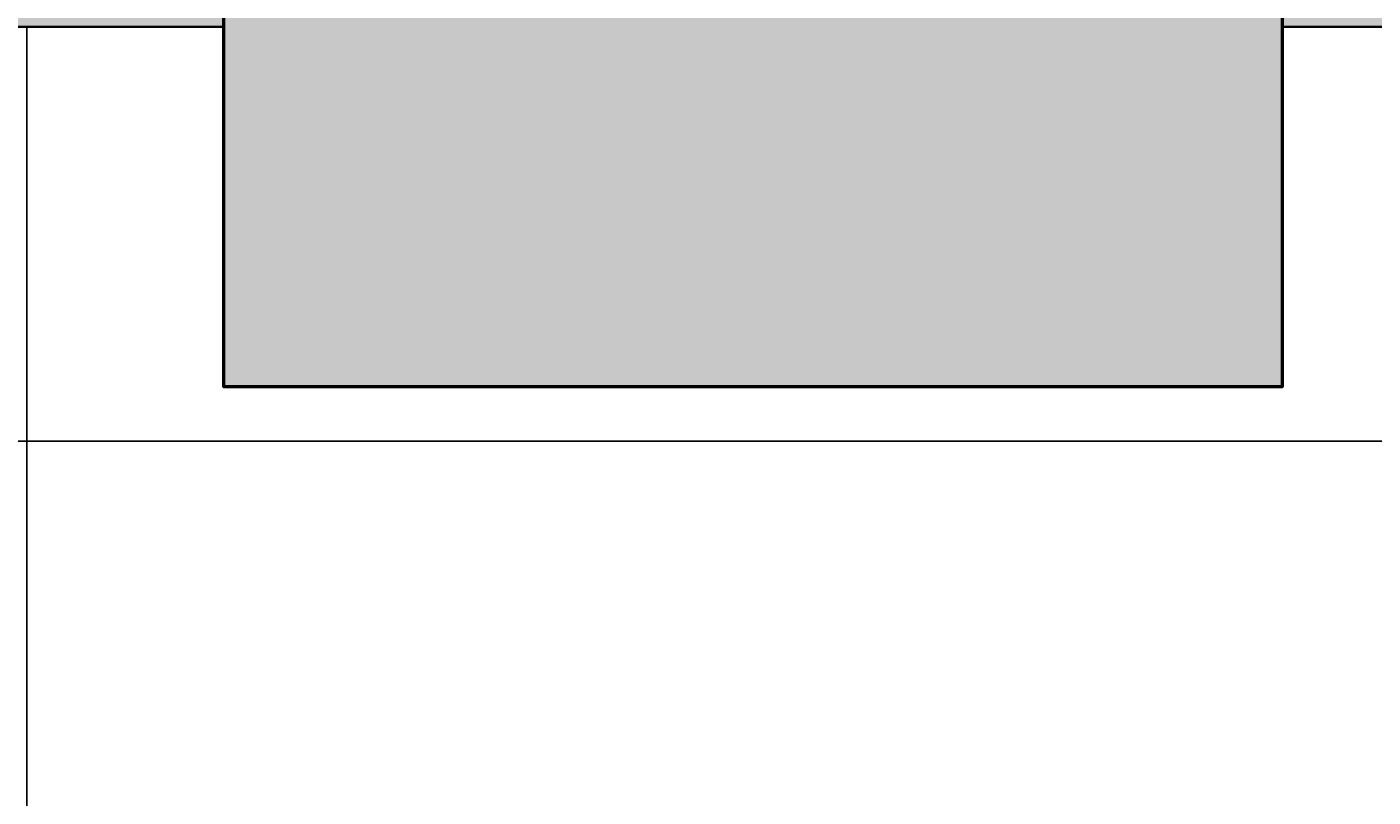
# Model space of a CAD drawing. Units: inches. Extents: x 1998 to 2588, y 1139 to 1977.
# Tile 119 of 134: x 2498 to 2524, y 1622 to 1637. Entities that reach past the tile are written whole.
import ezdxf

# ---------------------------------------------------------------- set-up
doc = ezdxf.new("R2010")
doc.units = ezdxf.units.IN
for name, color, linetype, lineweight in [('A-ANNO-DIMS', 2, 'Continuous', 18), ('A-COLS-PATT', 250, 'Continuous', 13), ('A-FLOR-STRS', 7, 'Continuous', 25), ('A-WALL-PATT', 252, 'Continuous', 13), ('COLUMN', 10, 'Continuous', 50), ('WALL', 200, 'Continuous', 35)]:
    doc.layers.add(name, color=color, linetype=linetype, lineweight=lineweight)
doc.styles.get("Standard").update_dxf_attribs({"font": 'arial.ttf'})
doc.dimstyles.get("Standard").update_dxf_attribs({"dimtxt": 0.18, "dimasz": 0.18, "dimexe": 0.18, "dimexo": 0.0625, "dimgap": 0.09, "dimtad": 0, "dimtih": 1, "dimtoh": 1, "dimdec": 4, "dimzin": 0, "dimdsep": 46, "dimtxsty": 'Standard', "dimcen": 0.09, "dimadec": 0, "dimazin": 0, "dimtfac": 1, "dimtdec": 4, "dimtofl": 0, "dimtmove": 0, "dimatfit": 3, "dimfxl": 1, "dimtolj": 1, "dimtzin": 0, "dimarcsym": 0})

# ---------------------------------------------------------------- blocks, each defined once
blk = doc.blocks.new('*D24')
at = {"layer": 'A-ANNO-DIMS', "color": 0, "lineweight": -2, "transparency": 16777216}
for p, q in [((2398.535, 1911.232), (2588.309, 1911.232)), ((2588.129, 1911.052), (2588.129, 1570.164)), ((2588.129, 1228.912), (2588.129, 1569.8)), ((2527.535, 1228.732), (2588.309, 1228.732))]:
    blk.add_line(p, q, dxfattribs=at)
at = {"layer": 'A-ANNO-DIMS', "color": 0, "transparency": 16777216}
for points in [[(2588.099, 1911.052), (2588.159, 1911.052), (2588.129, 1911.232)], [(2588.099, 1228.912), (2588.159, 1228.912), (2588.129, 1228.732)]]:
    blk.add_solid(points, dxfattribs=at)
at = {"layer": 'Defpoints', "color": 0, "transparency": 16777216}
for p in [(2398.473, 1911.232), (2588.129, 1911.232), (2527.473, 1228.732)]:
    blk.add_point(p, dxfattribs=at)
at = {"layer": 'A-ANNO-DIMS', "color": 0, "transparency": 16777216, "insert": (2588.129, 1569.982), "char_height": 0.18, "attachment_point": 5}
blk.add_mtext('\\A1;682.5', dxfattribs=at)
blk = doc.blocks.new('*D39')
at = {"layer": 'A-ANNO-DIMS', "color": 0, "lineweight": -2, "transparency": 16777216}
for p, q in [((2115.035, 1628.742), (2588.309, 1628.742)), ((2588.129, 1628.562), (2588.129, 1612.685)), ((2588.129, 1596.444), (2588.129, 1612.321)), ((2115.035, 1596.264), (2588.309, 1596.264))]:
    blk.add_line(p, q, dxfattribs=at)
at = {"layer": 'A-ANNO-DIMS', "color": 0, "transparency": 16777216}
for points in [[(2588.099, 1628.562), (2588.159, 1628.562), (2588.129, 1628.742)], [(2588.099, 1596.444), (2588.159, 1596.444), (2588.129, 1596.264)]]:
    blk.add_solid(points, dxfattribs=at)
at = {"layer": 'Defpoints', "color": 0, "transparency": 16777216}
for p in [(2114.973, 1628.742), (2588.129, 1628.742), (2114.973, 1596.264)]:
    blk.add_point(p, dxfattribs=at)
at = {"layer": 'A-ANNO-DIMS', "color": 0, "transparency": 16777216, "insert": (2588.129, 1612.503), "char_height": 0.18, "attachment_point": 5}
blk.add_mtext('\\A1;32.48', dxfattribs=at)

msp = doc.modelspace()

# ---------------------------------------------------------------- hatches: boundary and pattern name
at = {"layer": 'A-COLS-PATT'}
h = msp.add_hatch(color=256, dxfattribs=at)
h.dxf.hatch_style = 1
h.paths.add_polyline_path([(2099.4125, 1888.7324), (2087.9729, 1888.7324), (2087.9729, 1868.3278), (2099.4125, 1868.3278)])
h.paths.add_polyline_path([(2234.4125, 1888.7324), (2222.9729, 1888.7324), (2222.9729, 1868.3278), (2234.4125, 1868.3278)])
h.paths.add_polyline_path([(2341.4729, 1886.637), (2330.0332, 1886.637), (2330.0332, 1866.2324), (2341.4729, 1866.2324)])
h.paths.add_polyline_path([(2507.8006, 1882.7324), (2487.396, 1882.7324), (2487.396, 1871.2927), (2507.8006, 1871.2927)])
h.paths.add_polyline_path([(2510.9729, 1766.672), (2490.5682, 1766.672), (2490.5682, 1755.2324), (2510.9729, 1755.2324)])
h.paths.add_polyline_path([(2345.9729, 1759.7324), (2334.5332, 1759.7324), (2334.5332, 1739.3278), (2345.9729, 1739.3278)])
h.paths.add_polyline_path([(2234.4125, 1774.3318), (2222.9729, 1774.3318), (2222.9729, 1753.9272), (2234.4125, 1753.9272)])
h.paths.add_polyline_path([(2099.4125, 1775.637), (2087.9729, 1775.637), (2087.9729, 1755.2324), (2099.4125, 1755.2324)])
h.paths.add_polyline_path([(2098.0956, 1593.7241), (2077.691, 1593.7241), (2077.691, 1582.2845), (2098.0956, 1582.2845)])
h.paths.add_polyline_path([(2227.4729, 1604.637), (2216.0332, 1604.637), (2216.0332, 1584.2324), (2227.4729, 1584.2324)])
h.paths.add_polyline_path([(2345.9729, 1647.5211), (2334.5332, 1647.5211), (2334.5332, 1627.1165), (2345.9729, 1627.1165)])
h.paths.add_polyline_path([(2522.3775, 1641.2324), (2501.9729, 1641.2324), (2501.9729, 1629.7927), (2522.3775, 1629.7927)])
h.paths.add_polyline_path([(2522.3775, 1480.7324), (2501.9729, 1480.7324), (2501.9729, 1469.2927), (2522.3775, 1469.2927)])
h.paths.add_polyline_path([(2345.9729, 1488.5616), (2334.5332, 1488.5616), (2334.5332, 1468.1569), (2345.9729, 1468.1569)])
h.paths.add_polyline_path([(2234.4125, 1486.137), (2227.4729, 1486.137), (2227.4729, 1465.7324), (2234.4125, 1465.7324)])
h.paths.add_polyline_path([(2227.4729, 1486.137), (2222.9729, 1486.137), (2222.9729, 1465.7324), (2227.4729, 1465.7324)])
h.paths.add_polyline_path([(2108.3775, 1470.2324), (2087.9729, 1470.2324), (2087.9729, 1458.7927), (2108.3775, 1458.7927)])
h.paths.add_polyline_path([(2096.9729, 1365.5012), (2087.9729, 1365.5012), (2087.9729, 1345.0966), (2096.9729, 1345.0966)])
h.paths.add_polyline_path([(2087.9729, 1365.5012), (2085.5332, 1365.5012), (2085.5332, 1345.0966), (2087.9729, 1345.0966)])
h.paths.add_polyline_path([(2234.4125, 1285.137), (2222.9729, 1285.137), (2222.9729, 1264.7324), (2234.4125, 1264.7324)])
h.paths.add_polyline_path([(2345.9729, 1285.137), (2334.5332, 1285.137), (2334.5332, 1264.7324), (2345.9729, 1264.7324)])
h.paths.add_polyline_path([(2503.1458, 1240.172), (2482.7412, 1240.172), (2482.7412, 1228.7324), (2503.1458, 1228.7324)])
h.paths.add_polyline_path([(2510.9729, 1369.172), (2490.5682, 1369.172), (2490.5682, 1357.7324), (2510.9729, 1357.7324)])
at = {"layer": 'A-WALL-PATT'}
h = msp.add_hatch(color=256, dxfattribs=at)
h.dxf.hatch_style = 1
h.paths.add_polyline_path([(2527.4729, 1362.2324), (2510.9729, 1362.2324), (2510.9729, 1357.7324), (2518.4729, 1357.7324), (2518.4729, 1237.7324), (2503.1458, 1237.7324), (2503.1458, 1228.7324), (2527.4729, 1228.7324)])
h.paths.add_polyline_path([(2490.5682, 1362.2324), (2398.4729, 1362.2324), (2398.4729, 1357.7324), (2490.5682, 1357.7324)])
h.paths.add_polyline_path([(2224.9729, 1264.7324), (2222.9729, 1264.7324), (2222.9729, 1232.4125), (2341.4729, 1232.4125), (2341.4729, 1234.4125), (2224.9729, 1234.4125)])
h.paths.add_polyline_path([(2334.5332, 1273.7324), (2264.7638, 1273.7324), (2264.7638, 1269.5611, -0.043659), (2264.3413, 1264.7324), (2334.5332, 1264.7324)])
h.paths.add_polyline_path([(2236.9551, 1273.7324), (2234.4125, 1273.7324), (2234.4125, 1264.7324), (2236.9551, 1264.7324), (2236.9551, 1269.5611)])
h.paths.add_polyline_path([(2222.9729, 1293.2324), (2096.9729, 1293.2324), (2096.9729, 1345.0966), (2087.9729, 1345.0966), (2087.9729, 1284.2324), (2222.9729, 1284.2324), (2222.9729, 1285.137)])
h.paths.add_polyline_path([(2096.9729, 1458.7927), (2087.9729, 1458.7927), (2087.9729, 1417.7324), (2087.9729, 1413.2324), (2096.9729, 1413.2324), (2096.9729, 1417.7324)])
h.paths.add_polyline_path([(2096.9729, 1413.2324), (2087.9729, 1413.2324), (2087.9729, 1365.5012), (2096.9729, 1365.5012), (2096.9729, 1369.3358)])
h.paths.add_polyline_path([(2186.2943, 1417.7324), (2138.6074, 1417.7324), (2096.9729, 1417.7324), (2096.9729, 1413.2324), (2138.6074, 1413.2324), (2186.2943, 1413.2324)])
h.paths.add_polyline_path([(2181.4729, 1465.7324), (2176.9729, 1465.7324), (2176.9729, 1451.6434), (2181.4729, 1451.6434)])
h.paths.add_polyline_path([(2181.4729, 1422.1664), (2176.9729, 1422.1664), (2176.9729, 1417.7324), (2181.4729, 1417.7324)])
h.paths.add_polyline_path([(2063.9729, 1465.7324), (2087.9729, 1465.7324), (2087.9729, 1470.2324), (2059.4729, 1470.2324), (2059.4729, 1413.2324), (2087.9729, 1413.2324), (2087.9729, 1417.7324), (2063.9729, 1417.7324)])
h.paths.add_polyline_path([(2181.4729, 1755.2324), (2176.9729, 1755.2324), (2176.9729, 1748.6798), (2177.0513, 1748.6798), (2181.4729, 1748.6798)])
h.paths.add_polyline_path([(2227.4729, 1707.2324), (2220.4647, 1707.2324), (2220.4647, 1702.7324), (2222.9729, 1702.7324), (2222.9729, 1604.637), (2227.4729, 1604.637)])
h.paths.add_polyline_path([(2114.9729, 1702.7324), (2105.9729, 1702.7324), (2105.9729, 1628.4781, -0.0318759), (2110.1012, 1628.7416), (2114.9729, 1628.7416)])
h.paths.add_polyline_path([(2345.9729, 1739.3278), (2341.4729, 1739.3278), (2341.4729, 1647.5211), (2345.9729, 1647.5211)])
h.paths.add_polyline_path([(2350.6273, 1641.2324), (2345.9729, 1641.2324), (2345.9729, 1636.7324), (2350.6273, 1636.7324), (2350.6273, 1639.8729)])
h.paths.add_polyline_path([(2501.9729, 1641.2324), (2407.9729, 1641.2324), (2392.5005, 1641.2324), (2392.5005, 1639.8729), (2392.5005, 1636.7324), (2501.9729, 1636.7324)])
h.paths.add_polyline_path([(2510.9729, 1755.2324), (2501.9729, 1755.2324), (2501.9729, 1641.2324), (2510.9729, 1641.2324)])
h.paths.add_polyline_path([(2549.1786, 1641.2324), (2522.3775, 1641.2324), (2522.3775, 1636.7324), (2540.1786, 1636.7324), (2540.1786, 1480.7324), (2522.3775, 1480.7324), (2522.3775, 1476.2324), (2549.1786, 1476.2324)])
h.paths.add_polyline_path([(2498.1786, 1594.7324), (2407.9729, 1594.7324), (2407.9729, 1585.7324), (2416.9729, 1585.7324), (2489.1786, 1585.7324), (2489.1786, 1531.7324), (2416.9729, 1531.7324), (2407.9729, 1531.7324), (2407.9729, 1522.7324), (2498.1786, 1522.7324)])
h.paths.add_polyline_path([(2351.6437, 1480.7324), (2345.9729, 1480.7324), (2345.9729, 1476.2324), (2351.6437, 1476.2324), (2351.6437, 1477.5919)])
h.paths.add_polyline_path([(2501.9729, 1480.7324), (2498.1786, 1480.7324), (2407.9729, 1480.7324), (2393.5168, 1480.7324), (2393.5168, 1477.5919), (2393.5168, 1476.2324), (2501.9729, 1476.2324)])

# ---------------------------------------------------------------- linework, layer by layer
at = {"layer": 'A-FLOR-STRS'}
msp.add_line((2498.1786, 1480.7324), (2498.1786, 1636.7324), dxfattribs=at)
at = {"layer": 'COLUMN'}
msp.add_lwpolyline([(2522.3775, 1641.2324), (2522.3775, 1629.7927), (2501.9729, 1629.7927), (2501.9729, 1641.2324)], close=True, dxfattribs=at)
at = {"layer": 'WALL'}
for p, q in [((2501.9729, 1636.7324), (2392.5005, 1636.7324)), ((2407.9729, 1636.7324), (2501.9729, 1636.7324)), ((2501.9729, 1636.7324), (2498.1786, 1636.7324)), ((2540.1786, 1636.7324), (2522.3775, 1636.7324)), ((2522.3775, 1636.7324), (2540.1786, 1636.7324))]:
    msp.add_line(p, q, dxfattribs=at)

# ---------------------------------------------------------------- dimensions: what is measured, and where the dimension line sits
at = {"layer": 'A-ANNO-DIMS'}
for base, p1, p2, override, picture, middle in [((2588.1286, 1911.2324), (2527.4729, 1228.7324), (2398.4729, 1911.2324), {"dimdec": 1, "dimlfac": 1, "dimrnd": 0, "dimzin": 0, "dimdsep": 46, "dimlunit": 2}, '*D24', (2588.1286, 1569.9824)), ((2588.1286, 1628.7416), (2114.9729, 1596.2642), (2114.9729, 1628.7416), {"dimdec": 2, "dimlfac": 1, "dimrnd": 0, "dimzin": 0, "dimdsep": 46, "dimlunit": 2}, '*D39', (2588.1286, 1612.5029))]:
    dim = msp.add_linear_dim(base=base, p1=p1, p2=p2, angle=90, dimstyle='Standard', override=override, dxfattribs=at)
    dim.commit()
    dim.dimension.update_dxf_attribs({"geometry": picture, "text_midpoint": middle})

doc.saveas('drawing.dxf')
